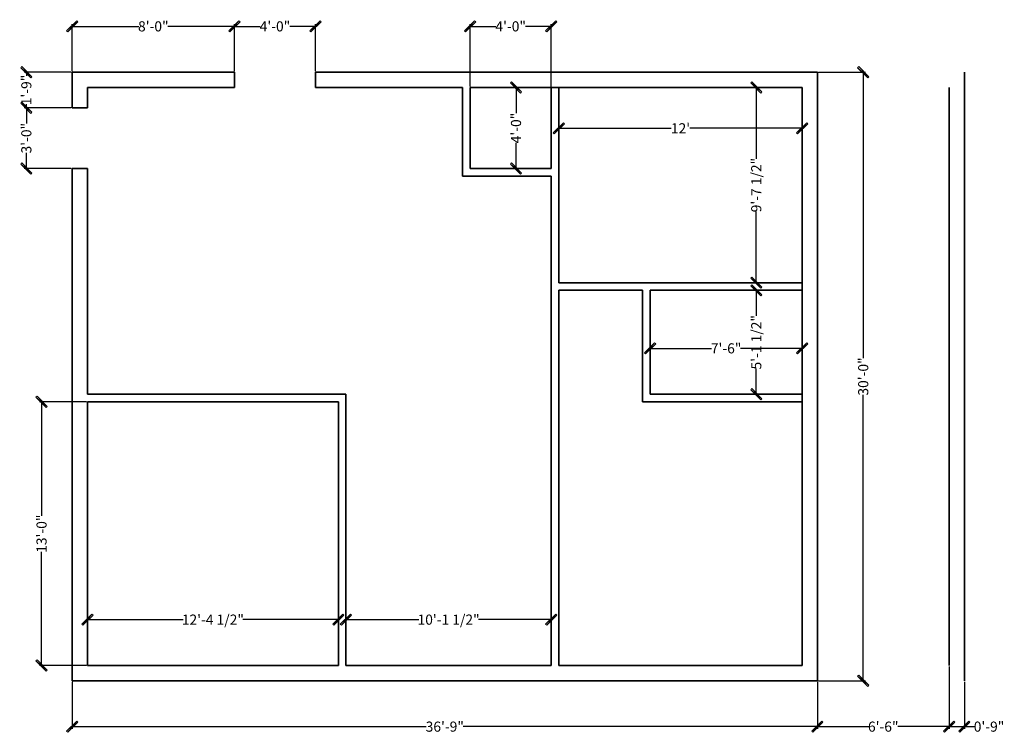
# Model space of a CAD drawing. Units: inches. Extents: x 1018 to 2596, y 723 to 1501.
# Tile 6 of 6: x 2014 to 2596, y 963 to 1385. Entities that reach past the tile are written whole.
import ezdxf

# ---------------------------------------------------------------- set-up
doc = ezdxf.new("R2010")
doc.units = ezdxf.units.IN
doc.layers.get('Defpoints').update_dxf_attribs({"lineweight": 0})
doc.layers.add('A-ANNO-DIMS', color=2, linetype='Continuous', lineweight=13)
doc.layers.add('A-WALL', color=7, linetype='Continuous', lineweight=35)
doc.styles.get("Standard").update_dxf_attribs({"font": 'arial.ttf'})
doc.dimstyles.new('saketh', dxfattribs={"dimtxt": 6, "dimasz": 6, "dimexe": 1.25, "dimexo": 0.625, "dimtad": 0, "dimdec": 1, "dimlunit": 4, "dimtxsty": 'Standard', "dimblk": 'ARCHTICK', "dimcen": 2.5, "dimclrd": 256, "dimclre": 1, "dimadec": 0, "dimazin": 0, "dimtfac": 1, "dimtdec": 1, "dimtmove": 0, "dimatfit": 3, "dimldrblk": 'ARCHTICK', "dimfxl": 1, "dimtolj": 1, "dimarcsym": 0})

# ---------------------------------------------------------------- blocks, each defined once
blk = doc.blocks.new('_ArchTick')
for p, q in [((0.447, 0.553), (-0.553, -0.447)), ((-0.447, -0.553), (0.553, 0.447)), ((0.553, 0.447), (0.447, 0.553)), ((-0.553, -0.447), (-0.447, -0.553))]:
    blk.add_line(p, q)
mesh = blk.add_polyface()
corners = [(-0.447, -0.553), (0.447, 0.553), (-0.553, -0.447), (0.553, 0.447)]
mesh.append_faces([[corners[k] for k in face] for face in [(0, 1, 2), (1, 0, 3)]], dxfattribs={"vtx0": -1})
blk = doc.blocks.new('*D2')
at = {"layer": 'A-ANNO-DIMS', "color": 0, "lineweight": -2, "transparency": 16777216}
for p, q in [((2332.82, 1327.95), (2332.82, 1319.31)), ((2476.82, 1327.95), (2476.82, 1319.31)), ((2332.82, 1320.56), (2399.39, 1320.56)), ((2476.82, 1320.56), (2410.26, 1320.56))]:
    blk.add_line(p, q, dxfattribs=at)
at = {"layer": 'Defpoints', "color": 0, "transparency": 16777216}
for p in [(2332.82, 1328.58), (2476.82, 1328.58), (2476.82, 1320.56)]:
    blk.add_point(p, dxfattribs=at)
at = {"layer": 'A-ANNO-DIMS', "color": 0, "lineweight": -2, "transparency": 16777216, "xscale": 6, "yscale": 6, "zscale": 6, "rotation": 180}
blk.add_blockref('_ArchTick', (2332.82, 1320.56), dxfattribs=at)
at = {"layer": 'A-ANNO-DIMS', "color": 0, "lineweight": -2, "transparency": 16777216, "xscale": 6, "yscale": 6, "zscale": 6}
blk.add_blockref('_ArchTick', (2476.82, 1320.56), dxfattribs=at)
at = {"layer": 'A-ANNO-DIMS', "color": 0, "transparency": 16777216, "insert": (2404.82, 1320.56), "char_height": 6, "attachment_point": 5}
blk.add_mtext("\\A1;12'", dxfattribs=at)
blk = doc.blocks.new('*D99')
at = {"layer": 'A-ANNO-DIMS', "color": 1, "lineweight": -2, "transparency": 16777216}
for p, q in [((2044.82, 993.1), (2044.82, 965.33)), ((2485.82, 993.1), (2485.82, 965.33))]:
    blk.add_line(p, q, dxfattribs=at)
at = {"layer": 'A-ANNO-DIMS', "lineweight": -2, "transparency": 16777216}
for p, q in [((2044.82, 966.58), (2254.4, 966.58)), ((2485.82, 966.58), (2276.25, 966.58))]:
    blk.add_line(p, q, dxfattribs=at)
at = {"layer": 'Defpoints', "color": 0, "transparency": 16777216}
for p in [(2044.82, 993.73), (2485.82, 993.73), (2485.82, 966.58)]:
    blk.add_point(p, dxfattribs=at)
at = {"layer": 'A-ANNO-DIMS', "lineweight": -2, "transparency": 16777216, "xscale": 6, "yscale": 6, "zscale": 6, "rotation": 180}
blk.add_blockref('_ArchTick', (2044.82, 966.58), dxfattribs=at)
at = {"layer": 'A-ANNO-DIMS', "lineweight": -2, "transparency": 16777216, "xscale": 6, "yscale": 6, "zscale": 6}
blk.add_blockref('_ArchTick', (2485.82, 966.58), dxfattribs=at)
at = {"layer": 'A-ANNO-DIMS', "color": 0, "transparency": 16777216, "insert": (2265.32, 966.58), "char_height": 6, "attachment_point": 5}
blk.add_mtext('\\A1;36\'-9"', dxfattribs=at)
blk = doc.blocks.new('*D100')
at = {"layer": 'A-ANNO-DIMS', "color": 1, "lineweight": -2, "transparency": 16777216}
for p, q in [((2486.45, 1353.73), (2514.22, 1353.73)), ((2486.45, 993.73), (2514.22, 993.73))]:
    blk.add_line(p, q, dxfattribs=at)
at = {"layer": 'A-ANNO-DIMS', "lineweight": -2, "transparency": 16777216}
for p, q in [((2512.97, 1353.73), (2512.97, 1184.65)), ((2512.97, 993.73), (2512.97, 1162.8))]:
    blk.add_line(p, q, dxfattribs=at)
at = {"layer": 'Defpoints', "color": 0, "transparency": 16777216}
for p in [(2485.82, 1353.73), (2485.82, 993.73), (2512.97, 993.73)]:
    blk.add_point(p, dxfattribs=at)
at = {"layer": 'A-ANNO-DIMS', "lineweight": -2, "transparency": 16777216, "xscale": 6, "yscale": 6, "zscale": 6}
for p, rotation in [((2512.97, 1353.73), 90), ((2512.97, 993.73), 270)]:
    blk.add_blockref('_ArchTick', p, dxfattribs=dict(at, rotation=rotation))
at = {"layer": 'A-ANNO-DIMS', "color": 0, "transparency": 16777216, "insert": (2512.97, 1173.73), "char_height": 6, "attachment_point": 5, "rotation": 90}
blk.add_mtext('\\A1;30\'-0"', dxfattribs=at)
blk = doc.blocks.new('*D101')
at = {"layer": 'A-ANNO-DIMS', "color": 1, "lineweight": -2, "transparency": 16777216}
for p, q in [((2053.82, 1003.35), (2053.82, 1031.13)), ((2202.32, 1003.35), (2202.32, 1031.13))]:
    blk.add_line(p, q, dxfattribs=at)
at = {"layer": 'A-ANNO-DIMS', "lineweight": -2, "transparency": 16777216}
for p, q in [((2053.82, 1029.88), (2110.44, 1029.88)), ((2202.32, 1029.88), (2145.71, 1029.88))]:
    blk.add_line(p, q, dxfattribs=at)
at = {"layer": 'Defpoints', "color": 0, "transparency": 16777216}
for p in [(2202.32, 1029.88), (2053.82, 1002.73), (2202.32, 1002.73)]:
    blk.add_point(p, dxfattribs=at)
at = {"layer": 'A-ANNO-DIMS', "lineweight": -2, "transparency": 16777216, "xscale": 6, "yscale": 6, "zscale": 6, "rotation": 180}
blk.add_blockref('_ArchTick', (2053.82, 1029.88), dxfattribs=at)
at = {"layer": 'A-ANNO-DIMS', "lineweight": -2, "transparency": 16777216, "xscale": 6, "yscale": 6, "zscale": 6}
blk.add_blockref('_ArchTick', (2202.32, 1029.88), dxfattribs=at)
at = {"layer": 'A-ANNO-DIMS', "color": 0, "transparency": 16777216, "insert": (2128.07, 1029.88), "char_height": 6, "attachment_point": 5}
blk.add_mtext('\\A1;12\'-4 1/2"', dxfattribs=at)
blk = doc.blocks.new('*D102')
at = {"layer": 'A-ANNO-DIMS', "color": 1, "lineweight": -2, "transparency": 16777216}
for p, q in [((2053.2, 1158.73), (2025.42, 1158.73)), ((2053.2, 1002.73), (2025.42, 1002.73))]:
    blk.add_line(p, q, dxfattribs=at)
at = {"layer": 'A-ANNO-DIMS', "lineweight": -2, "transparency": 16777216}
for p, q in [((2026.67, 1158.73), (2026.67, 1091.37)), ((2026.67, 1002.73), (2026.67, 1070.08))]:
    blk.add_line(p, q, dxfattribs=at)
at = {"layer": 'Defpoints', "color": 0, "transparency": 16777216}
for p in [(2026.67, 1158.73), (2053.82, 1158.73), (2053.82, 1002.73)]:
    blk.add_point(p, dxfattribs=at)
at = {"layer": 'A-ANNO-DIMS', "lineweight": -2, "transparency": 16777216, "xscale": 6, "yscale": 6, "zscale": 6}
for p, rotation in [((2026.67, 1158.73), 90), ((2026.67, 1002.73), 270)]:
    blk.add_blockref('_ArchTick', p, dxfattribs=dict(at, rotation=rotation))
at = {"layer": 'A-ANNO-DIMS', "color": 0, "transparency": 16777216, "insert": (2026.67, 1080.73), "char_height": 6, "attachment_point": 5, "rotation": 90}
blk.add_mtext('\\A1;13\'-0"', dxfattribs=at)
blk = doc.blocks.new('*D103')
at = {"layer": 'A-ANNO-DIMS', "color": 1, "lineweight": -2, "transparency": 16777216}
for p, q in [((2280.32, 1345.35), (2280.32, 1382.13)), ((2328.32, 1345.35), (2328.32, 1382.13))]:
    blk.add_line(p, q, dxfattribs=at)
at = {"layer": 'A-ANNO-DIMS', "lineweight": -2, "transparency": 16777216}
for p, q in [((2280.32, 1380.88), (2295.6, 1380.88)), ((2328.32, 1380.88), (2313.04, 1380.88))]:
    blk.add_line(p, q, dxfattribs=at)
at = {"layer": 'Defpoints', "color": 0, "transparency": 16777216}
for p in [(2328.32, 1380.88), (2280.32, 1344.73), (2328.32, 1344.73)]:
    blk.add_point(p, dxfattribs=at)
at = {"layer": 'A-ANNO-DIMS', "lineweight": -2, "transparency": 16777216, "xscale": 6, "yscale": 6, "zscale": 6, "rotation": 180}
blk.add_blockref('_ArchTick', (2280.32, 1380.88), dxfattribs=at)
at = {"layer": 'A-ANNO-DIMS', "lineweight": -2, "transparency": 16777216, "xscale": 6, "yscale": 6, "zscale": 6}
blk.add_blockref('_ArchTick', (2328.32, 1380.88), dxfattribs=at)
at = {"layer": 'A-ANNO-DIMS', "color": 0, "transparency": 16777216, "insert": (2304.32, 1380.88), "char_height": 6, "attachment_point": 5}
blk.add_mtext('\\A1;4\'-0"', dxfattribs=at)
blk = doc.blocks.new('*D104')
at = {"layer": 'A-ANNO-DIMS', "color": 1, "lineweight": -2, "transparency": 16777216}
for p, q in [((2280.95, 1344.73), (2308.72, 1344.73)), ((2280.95, 1296.73), (2308.72, 1296.73))]:
    blk.add_line(p, q, dxfattribs=at)
at = {"layer": 'A-ANNO-DIMS', "lineweight": -2, "transparency": 16777216}
for p, q in [((2307.47, 1344.73), (2307.47, 1329.45)), ((2307.47, 1296.73), (2307.47, 1312))]:
    blk.add_line(p, q, dxfattribs=at)
at = {"layer": 'Defpoints', "color": 0, "transparency": 16777216}
for p in [(2280.32, 1344.73), (2280.32, 1296.73), (2307.47, 1296.73)]:
    blk.add_point(p, dxfattribs=at)
at = {"layer": 'A-ANNO-DIMS', "lineweight": -2, "transparency": 16777216, "xscale": 6, "yscale": 6, "zscale": 6}
for p, rotation in [((2307.47, 1344.73), 90), ((2307.47, 1296.73), 270)]:
    blk.add_blockref('_ArchTick', p, dxfattribs=dict(at, rotation=rotation))
at = {"layer": 'A-ANNO-DIMS', "color": 0, "transparency": 16777216, "insert": (2307.47, 1320.73), "char_height": 6, "attachment_point": 5, "rotation": 90}
blk.add_mtext('\\A1;4\'-0"', dxfattribs=at)
blk = doc.blocks.new('*D105')
at = {"layer": 'A-ANNO-DIMS', "color": 1, "lineweight": -2, "transparency": 16777216}
for p, q in [((2476.2, 1344.73), (2448.42, 1344.73)), ((2476.2, 1229.23), (2448.42, 1229.23))]:
    blk.add_line(p, q, dxfattribs=at)
at = {"layer": 'A-ANNO-DIMS', "lineweight": -2, "transparency": 16777216}
for p, q in [((2449.67, 1344.73), (2449.67, 1302.57)), ((2449.67, 1229.23), (2449.67, 1271.39))]:
    blk.add_line(p, q, dxfattribs=at)
at = {"layer": 'Defpoints', "color": 0, "transparency": 16777216}
for p in [(2449.67, 1344.73), (2476.82, 1344.73), (2476.82, 1229.23)]:
    blk.add_point(p, dxfattribs=at)
at = {"layer": 'A-ANNO-DIMS', "lineweight": -2, "transparency": 16777216, "xscale": 6, "yscale": 6, "zscale": 6}
for p, rotation in [((2449.67, 1344.73), 90), ((2449.67, 1229.23), 270)]:
    blk.add_blockref('_ArchTick', p, dxfattribs=dict(at, rotation=rotation))
at = {"layer": 'A-ANNO-DIMS', "color": 0, "transparency": 16777216, "insert": (2449.67, 1286.98), "char_height": 6, "attachment_point": 5, "rotation": 90}
blk.add_mtext('\\A1;9\'-7 1/2"', dxfattribs=at)
blk = doc.blocks.new('*D106')
at = {"layer": 'A-ANNO-DIMS', "color": 1, "lineweight": -2, "transparency": 16777216}
for p, q in [((2386.82, 1163.85), (2386.82, 1191.63)), ((2476.82, 1163.85), (2476.82, 1191.63))]:
    blk.add_line(p, q, dxfattribs=at)
at = {"layer": 'A-ANNO-DIMS', "lineweight": -2, "transparency": 16777216}
for p, q in [((2386.82, 1190.38), (2423.25, 1190.38)), ((2476.82, 1190.38), (2440.4, 1190.38))]:
    blk.add_line(p, q, dxfattribs=at)
at = {"layer": 'Defpoints', "color": 0, "transparency": 16777216}
for p in [(2476.82, 1190.38), (2386.82, 1163.23), (2476.82, 1163.23)]:
    blk.add_point(p, dxfattribs=at)
at = {"layer": 'A-ANNO-DIMS', "lineweight": -2, "transparency": 16777216, "xscale": 6, "yscale": 6, "zscale": 6, "rotation": 180}
blk.add_blockref('_ArchTick', (2386.82, 1190.38), dxfattribs=at)
at = {"layer": 'A-ANNO-DIMS', "lineweight": -2, "transparency": 16777216, "xscale": 6, "yscale": 6, "zscale": 6}
blk.add_blockref('_ArchTick', (2476.82, 1190.38), dxfattribs=at)
at = {"layer": 'A-ANNO-DIMS', "color": 0, "transparency": 16777216, "insert": (2431.82, 1190.38), "char_height": 6, "attachment_point": 5}
blk.add_mtext('\\A1;7\'-6"', dxfattribs=at)
blk = doc.blocks.new('*D107')
at = {"layer": 'A-ANNO-DIMS', "color": 1, "lineweight": -2, "transparency": 16777216}
for p, q in [((2476.2, 1224.73), (2448.42, 1224.73)), ((2476.2, 1163.23), (2448.42, 1163.23))]:
    blk.add_line(p, q, dxfattribs=at)
at = {"layer": 'A-ANNO-DIMS', "lineweight": -2, "transparency": 16777216}
for p, q in [((2449.67, 1224.73), (2449.67, 1209.57)), ((2449.67, 1163.23), (2449.67, 1178.39))]:
    blk.add_line(p, q, dxfattribs=at)
at = {"layer": 'Defpoints', "color": 0, "transparency": 16777216}
for p in [(2449.67, 1224.73), (2476.82, 1224.73), (2476.82, 1163.23)]:
    blk.add_point(p, dxfattribs=at)
at = {"layer": 'A-ANNO-DIMS', "lineweight": -2, "transparency": 16777216, "xscale": 6, "yscale": 6, "zscale": 6}
for p, rotation in [((2449.67, 1224.73), 90), ((2449.67, 1163.23), 270)]:
    blk.add_blockref('_ArchTick', p, dxfattribs=dict(at, rotation=rotation))
at = {"layer": 'A-ANNO-DIMS', "color": 0, "transparency": 16777216, "insert": (2449.67, 1193.98), "char_height": 6, "attachment_point": 5, "rotation": 90}
blk.add_mtext('\\A1;5\'-1 1/2"', dxfattribs=at)
blk = doc.blocks.new('*D108')
at = {"layer": 'A-ANNO-DIMS', "color": 1, "lineweight": -2, "transparency": 16777216}
for p, q in [((2206.82, 1003.35), (2206.82, 1031.13)), ((2328.32, 1003.35), (2328.32, 1031.13))]:
    blk.add_line(p, q, dxfattribs=at)
at = {"layer": 'A-ANNO-DIMS', "lineweight": -2, "transparency": 16777216}
for p, q in [((2206.82, 1029.88), (2249.94, 1029.88)), ((2328.32, 1029.88), (2285.21, 1029.88))]:
    blk.add_line(p, q, dxfattribs=at)
at = {"layer": 'Defpoints', "color": 0, "transparency": 16777216}
for p in [(2328.32, 1029.88), (2206.82, 1002.73), (2328.32, 1002.73)]:
    blk.add_point(p, dxfattribs=at)
at = {"layer": 'A-ANNO-DIMS', "lineweight": -2, "transparency": 16777216, "xscale": 6, "yscale": 6, "zscale": 6, "rotation": 180}
blk.add_blockref('_ArchTick', (2206.82, 1029.88), dxfattribs=at)
at = {"layer": 'A-ANNO-DIMS', "lineweight": -2, "transparency": 16777216, "xscale": 6, "yscale": 6, "zscale": 6}
blk.add_blockref('_ArchTick', (2328.32, 1029.88), dxfattribs=at)
at = {"layer": 'A-ANNO-DIMS', "color": 0, "transparency": 16777216, "insert": (2267.57, 1029.88), "char_height": 6, "attachment_point": 5}
blk.add_mtext('\\A1;10\'-1 1/2"', dxfattribs=at)
blk = doc.blocks.new('*D109')
at = {"layer": 'A-ANNO-DIMS', "color": 1, "lineweight": -2, "transparency": 16777216}
for p, q in [((2563.82, 1002.1), (2563.82, 965.33)), ((2485.82, 993.1), (2485.82, 965.33))]:
    blk.add_line(p, q, dxfattribs=at)
at = {"layer": 'A-ANNO-DIMS', "lineweight": -2, "transparency": 16777216}
for p, q in [((2485.82, 966.58), (2516.21, 966.58)), ((2563.82, 966.58), (2533.44, 966.58))]:
    blk.add_line(p, q, dxfattribs=at)
at = {"layer": 'Defpoints', "color": 0, "transparency": 16777216}
for p in [(2563.82, 1002.73), (2485.82, 993.73), (2563.82, 966.58)]:
    blk.add_point(p, dxfattribs=at)
at = {"layer": 'A-ANNO-DIMS', "lineweight": -2, "transparency": 16777216, "xscale": 6, "yscale": 6, "zscale": 6, "rotation": 180}
blk.add_blockref('_ArchTick', (2485.82, 966.58), dxfattribs=at)
at = {"layer": 'A-ANNO-DIMS', "lineweight": -2, "transparency": 16777216, "xscale": 6, "yscale": 6, "zscale": 6}
blk.add_blockref('_ArchTick', (2563.82, 966.58), dxfattribs=at)
at = {"layer": 'A-ANNO-DIMS', "color": 0, "transparency": 16777216, "insert": (2524.82, 966.58), "char_height": 6, "attachment_point": 5}
blk.add_mtext('\\A1;6\'-6"', dxfattribs=at)
blk = doc.blocks.new('*D110')
at = {"layer": 'A-ANNO-DIMS', "color": 1, "lineweight": -2, "transparency": 16777216}
for p, q in [((2563.82, 1002.1), (2563.82, 965.33)), ((2572.82, 993.1), (2572.82, 965.33))]:
    blk.add_line(p, q, dxfattribs=at)
at = {"layer": 'A-ANNO-DIMS', "lineweight": -2, "transparency": 16777216}
for p, q in [((2563.82, 966.58), (2572.82, 966.58)), ((2572.82, 966.58), (2578.82, 966.58))]:
    blk.add_line(p, q, dxfattribs=at)
at = {"layer": 'Defpoints', "color": 0, "transparency": 16777216}
for p in [(2563.82, 1002.73), (2572.82, 993.73), (2572.82, 966.58)]:
    blk.add_point(p, dxfattribs=at)
at = {"layer": 'A-ANNO-DIMS', "lineweight": -2, "transparency": 16777216, "xscale": 6, "yscale": 6, "zscale": 6, "rotation": 180}
blk.add_blockref('_ArchTick', (2563.82, 966.58), dxfattribs=at)
at = {"layer": 'A-ANNO-DIMS', "lineweight": -2, "transparency": 16777216, "xscale": 6, "yscale": 6, "zscale": 6}
blk.add_blockref('_ArchTick', (2572.82, 966.58), dxfattribs=at)
at = {"layer": 'A-ANNO-DIMS', "color": 0, "transparency": 16777216, "insert": (2587.42, 966.58), "char_height": 6, "attachment_point": 5}
blk.add_mtext('\\A1;0\'-9"', dxfattribs=at)
blk = doc.blocks.new('*D111')
at = {"layer": 'A-ANNO-DIMS', "color": 1, "lineweight": -2, "transparency": 16777216}
for p, q in [((2044.82, 1354.35), (2044.82, 1382.13)), ((2140.82, 1354.35), (2140.82, 1382.13))]:
    blk.add_line(p, q, dxfattribs=at)
at = {"layer": 'A-ANNO-DIMS', "lineweight": -2, "transparency": 16777216}
for p, q in [((2044.82, 1380.88), (2084.22, 1380.88)), ((2140.82, 1380.88), (2101.43, 1380.88))]:
    blk.add_line(p, q, dxfattribs=at)
at = {"layer": 'Defpoints', "color": 0, "transparency": 16777216}
for p in [(2140.82, 1380.88), (2044.82, 1353.73), (2140.82, 1353.73)]:
    blk.add_point(p, dxfattribs=at)
at = {"layer": 'A-ANNO-DIMS', "lineweight": -2, "transparency": 16777216, "xscale": 6, "yscale": 6, "zscale": 6, "rotation": 180}
blk.add_blockref('_ArchTick', (2044.82, 1380.88), dxfattribs=at)
at = {"layer": 'A-ANNO-DIMS', "lineweight": -2, "transparency": 16777216, "xscale": 6, "yscale": 6, "zscale": 6}
blk.add_blockref('_ArchTick', (2140.82, 1380.88), dxfattribs=at)
at = {"layer": 'A-ANNO-DIMS', "color": 0, "transparency": 16777216, "insert": (2092.82, 1380.88), "char_height": 6, "attachment_point": 5}
blk.add_mtext('\\A1;8\'-0"', dxfattribs=at)
blk = doc.blocks.new('*D112')
at = {"layer": 'A-ANNO-DIMS', "color": 1, "lineweight": -2, "transparency": 16777216}
for p, q in [((2140.82, 1354.35), (2140.82, 1382.13)), ((2188.82, 1354.35), (2188.82, 1382.13))]:
    blk.add_line(p, q, dxfattribs=at)
at = {"layer": 'A-ANNO-DIMS', "lineweight": -2, "transparency": 16777216}
for p, q in [((2140.82, 1380.88), (2156.1, 1380.88)), ((2188.82, 1380.88), (2173.54, 1380.88))]:
    blk.add_line(p, q, dxfattribs=at)
at = {"layer": 'Defpoints', "color": 0, "transparency": 16777216}
for p in [(2188.82, 1380.88), (2140.82, 1353.73), (2188.82, 1353.73)]:
    blk.add_point(p, dxfattribs=at)
at = {"layer": 'A-ANNO-DIMS', "lineweight": -2, "transparency": 16777216, "xscale": 6, "yscale": 6, "zscale": 6, "rotation": 180}
blk.add_blockref('_ArchTick', (2140.82, 1380.88), dxfattribs=at)
at = {"layer": 'A-ANNO-DIMS', "lineweight": -2, "transparency": 16777216, "xscale": 6, "yscale": 6, "zscale": 6}
blk.add_blockref('_ArchTick', (2188.82, 1380.88), dxfattribs=at)
at = {"layer": 'A-ANNO-DIMS', "color": 0, "transparency": 16777216, "insert": (2164.82, 1380.88), "char_height": 6, "attachment_point": 5}
blk.add_mtext('\\A1;4\'-0"', dxfattribs=at)
blk = doc.blocks.new('*D113')
at = {"layer": 'A-ANNO-DIMS', "color": 1, "lineweight": -2, "transparency": 16777216}
for p, q in [((2044.2, 1353.73), (2016.42, 1353.73)), ((2044.2, 1332.73), (2016.42, 1332.73))]:
    blk.add_line(p, q, dxfattribs=at)
at = {"layer": 'A-ANNO-DIMS', "lineweight": -2, "transparency": 16777216}
for p, q in [((2017.67, 1353.73), (2017.67, 1351.54)), ((2017.67, 1332.73), (2017.67, 1334.91))]:
    blk.add_line(p, q, dxfattribs=at)
at = {"layer": 'Defpoints', "color": 0, "transparency": 16777216}
for p in [(2044.82, 1353.73), (2017.67, 1332.73), (2044.82, 1332.73)]:
    blk.add_point(p, dxfattribs=at)
at = {"layer": 'A-ANNO-DIMS', "lineweight": -2, "transparency": 16777216, "xscale": 6, "yscale": 6, "zscale": 6}
for p, rotation in [((2017.67, 1353.73), 90), ((2017.67, 1332.73), 270)]:
    blk.add_blockref('_ArchTick', p, dxfattribs=dict(at, rotation=rotation))
at = {"layer": 'A-ANNO-DIMS', "color": 0, "transparency": 16777216, "insert": (2017.67, 1343.23), "char_height": 6, "attachment_point": 5, "rotation": 90}
blk.add_mtext('\\A1;1\'-9"', dxfattribs=at)
blk = doc.blocks.new('*D114')
at = {"layer": 'A-ANNO-DIMS', "color": 1, "lineweight": -2, "transparency": 16777216}
for p, q in [((2044.2, 1332.73), (2016.42, 1332.73)), ((2044.2, 1296.73), (2016.42, 1296.73))]:
    blk.add_line(p, q, dxfattribs=at)
at = {"layer": 'A-ANNO-DIMS', "lineweight": -2, "transparency": 16777216}
for p, q in [((2017.67, 1332.73), (2017.67, 1323.32)), ((2017.67, 1296.73), (2017.67, 1306.13))]:
    blk.add_line(p, q, dxfattribs=at)
at = {"layer": 'Defpoints', "color": 0, "transparency": 16777216}
for p in [(2044.82, 1332.73), (2017.67, 1296.73), (2044.82, 1296.73)]:
    blk.add_point(p, dxfattribs=at)
at = {"layer": 'A-ANNO-DIMS', "lineweight": -2, "transparency": 16777216, "xscale": 6, "yscale": 6, "zscale": 6}
for p, rotation in [((2017.67, 1332.73), 90), ((2017.67, 1296.73), 270)]:
    blk.add_blockref('_ArchTick', p, dxfattribs=dict(at, rotation=rotation))
at = {"layer": 'A-ANNO-DIMS', "color": 0, "transparency": 16777216, "insert": (2017.67, 1314.73), "char_height": 6, "attachment_point": 5, "rotation": 90}
blk.add_mtext('\\A1;3\'-0"', dxfattribs=at)

msp = doc.modelspace()

# ---------------------------------------------------------------- linework, layer by layer
at = {"layer": 'A-WALL'}
for p, q in [((2044.82, 1353.73), (2140.82, 1353.73)), ((2044.82, 1332.73), (2044.82, 1353.73)), ((2140.82, 1344.73), (2140.82, 1353.73)), ((2188.82, 1353.73), (2485.82, 1353.73)), ((2188.82, 1344.73), (2188.82, 1353.73)), ((2485.82, 1353.73), (2485.82, 993.73)), ((2572.82, 1353.73), (2572.82, 993.73)), ((2053.82, 1344.73), (2140.82, 1344.73)), ((2053.82, 1332.73), (2053.82, 1344.73)), ((2188.82, 1344.73), (2275.82, 1344.73)), ((2275.82, 1292.23), (2275.82, 1344.73)), ((2280.32, 1344.73), (2476.82, 1344.73)), ((2280.32, 1296.73), (2280.32, 1344.73)), ((2328.32, 1296.73), (2328.32, 1344.73)), ((2332.82, 1229.23), (2332.82, 1344.73)), ((2476.82, 1344.73), (2476.82, 1002.73)), ((2563.82, 1344.73), (2563.82, 1002.73)), ((2053.82, 1332.73), (2044.82, 1332.73)), ((2044.82, 993.73), (2044.82, 1296.73)), ((2053.82, 1296.73), (2044.82, 1296.73)), ((2053.82, 1163.23), (2053.82, 1296.73)), ((2280.32, 1296.73), (2328.32, 1296.73)), ((2275.82, 1292.23), (2328.32, 1292.23)), ((2328.32, 1229.23), (2328.32, 1292.23)), ((2328.32, 1229.23), (2328.32, 1002.73)), ((2332.82, 1229.23), (2476.82, 1229.23)), ((2332.82, 1224.73), (2382.32, 1224.73)), ((2332.82, 1224.73), (2332.82, 1002.73)), ((2382.32, 1224.73), (2382.32, 1158.73)), ((2386.82, 1224.73), (2476.82, 1224.73)), ((2386.82, 1224.73), (2386.82, 1163.23)), ((2206.82, 1163.23), (2053.82, 1163.23)), ((2206.82, 1163.23), (2206.82, 1002.73)), ((2476.82, 1163.23), (2386.82, 1163.23)), ((2202.32, 1158.73), (2053.82, 1158.73)), ((2053.82, 1002.73), (2053.82, 1158.73)), ((2202.32, 1158.73), (2202.32, 1002.73)), ((2476.82, 1158.73), (2382.32, 1158.73)), ((2202.32, 1002.73), (2053.82, 1002.73)), ((2328.32, 1002.73), (2206.82, 1002.73)), ((2476.82, 1002.73), (2332.82, 1002.73)), ((2485.82, 993.73), (2044.82, 993.73))]:
    msp.add_line(p, q, dxfattribs=at)

# ---------------------------------------------------------------- dimensions: what is measured, and where the dimension line sits
at = {"layer": 'A-ANNO-DIMS'}
for base, p1, p2, override, picture, middle in [((2140.82, 1380.88), (2044.82, 1353.73), (2140.82, 1353.73), {"dimdec": 1, "dimlfac": 1, "dimrnd": 0, "dimzin": 1, "dimdsep": 46, "dimlunit": 4, "dimfrac": 2}, '*D111', (2092.82, 1380.88)), ((2188.82, 1380.88), (2140.82, 1353.73), (2188.82, 1353.73), {"dimdec": 1, "dimlfac": 1, "dimrnd": 0, "dimzin": 1, "dimdsep": 46, "dimlunit": 4, "dimfrac": 2}, '*D112', (2164.82, 1380.88)), ((2328.32, 1380.88), (2280.32, 1344.73), (2328.32, 1344.73), {"dimdec": 1, "dimlfac": 1, "dimrnd": 0, "dimzin": 1, "dimdsep": 46, "dimlunit": 4, "dimfrac": 2}, '*D103', (2304.32, 1380.88)), ((2476.82, 1320.56), (2332.82, 1328.58), (2476.82, 1328.58), {"dimclrd": 0, "dimclre": 0, "dimclrt": 0}, '*D2', (2404.82, 1320.56)), ((2476.82, 1190.38), (2386.82, 1163.23), (2476.82, 1163.23), {"dimdec": 1, "dimlfac": 1, "dimrnd": 0, "dimzin": 1, "dimdsep": 46, "dimlunit": 4, "dimfrac": 2}, '*D106', (2431.82, 1190.38)), ((2202.32, 1029.88), (2053.82, 1002.73), (2202.32, 1002.73), {"dimdec": 1, "dimlfac": 1, "dimrnd": 0, "dimzin": 1, "dimdsep": 46, "dimlunit": 4, "dimfrac": 2}, '*D101', (2128.07, 1029.88)), ((2328.32, 1029.88), (2206.82, 1002.73), (2328.32, 1002.73), {"dimdec": 1, "dimlfac": 1, "dimrnd": 0, "dimzin": 1, "dimdsep": 46, "dimlunit": 4, "dimfrac": 2}, '*D108', (2267.57, 1029.88)), ((2563.82, 966.58), (2485.82, 993.73), (2563.82, 1002.73), {"dimdec": 1, "dimlfac": 1, "dimrnd": 0, "dimzin": 1, "dimdsep": 46, "dimlunit": 4, "dimfrac": 2}, '*D109', (2524.82, 966.58)), ((2572.82, 966.58), (2563.82, 1002.73), (2572.82, 993.73), {"dimdec": 1, "dimlfac": 1, "dimrnd": 0, "dimzin": 1, "dimdsep": 46, "dimlunit": 4, "dimfrac": 2}, '*D110', (2587.42, 966.58)), ((2485.82, 966.58), (2044.82, 993.73), (2485.82, 993.73), {"dimdec": 1, "dimlfac": 1, "dimrnd": 0, "dimzin": 1, "dimdsep": 46, "dimlunit": 4, "dimfrac": 2}, '*D99', (2265.32, 966.58))]:
    dim = msp.add_linear_dim(base=base, p1=p1, p2=p2, dimstyle='saketh', override=override, dxfattribs=at)
    dim.commit()
    dim.dimension.update_dxf_attribs({"geometry": picture, "text_midpoint": middle})
for base, p1, p2, angle, picture, middle in [((2017.67, 1332.73), (2044.82, 1353.73), (2044.82, 1332.73), 90, '*D113', (2017.67, 1343.23)), ((2512.97, 993.73), (2485.82, 1353.73), (2485.82, 993.73), 270, '*D100', (2512.97, 1173.73)), ((2307.47, 1296.73), (2280.32, 1344.73), (2280.32, 1296.73), 270, '*D104', (2307.47, 1320.73)), ((2449.67, 1344.73), (2476.82, 1229.23), (2476.82, 1344.73), 90, '*D105', (2449.67, 1286.98)), ((2017.67, 1296.73), (2044.82, 1332.73), (2044.82, 1296.73), 90, '*D114', (2017.67, 1314.73)), ((2449.67, 1224.73), (2476.82, 1163.23), (2476.82, 1224.73), 90, '*D107', (2449.67, 1193.98)), ((2026.67, 1158.73), (2053.82, 1002.73), (2053.82, 1158.73), 90, '*D102', (2026.67, 1080.73))]:
    dim = msp.add_linear_dim(base=base, p1=p1, p2=p2, angle=angle, dimstyle='saketh', override={"dimdec": 1, "dimlfac": 1, "dimrnd": 0, "dimzin": 1, "dimdsep": 46, "dimlunit": 4, "dimfrac": 2}, dxfattribs=at)
    dim.commit()
    dim.dimension.update_dxf_attribs({"geometry": picture, "text_midpoint": middle})

doc.saveas('drawing.dxf')
